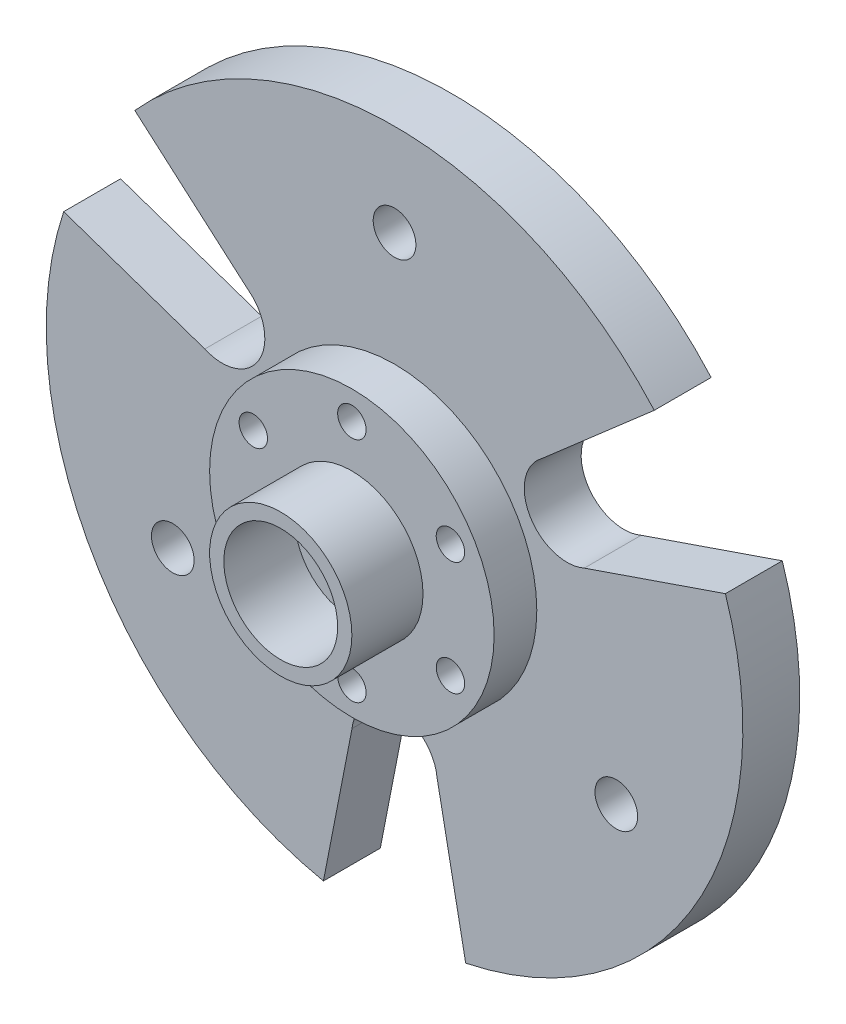
ISO-10303-21;
HEADER;
FILE_DESCRIPTION(('STEP AP214'),'2;1');
FILE_NAME('part.step','',(''),(''),'','','');
FILE_SCHEMA(('AUTOMOTIVE_DESIGN { 1 0 10303 214 1 1 1 1 }'));
ENDSEC;
DATA;
#1=APPLICATION_CONTEXT('core data for automotive mechanical design processes');
#2=APPLICATION_PROTOCOL_DEFINITION('international standard','automotive_design',2000,#1);
#3=PRODUCT_CONTEXT('',#1,'mechanical');
#4=PRODUCT('Part','Part','',(#3));
#5=PRODUCT_RELATED_PRODUCT_CATEGORY('part','',(#4));
#6=PRODUCT_DEFINITION_FORMATION('','',#4);
#7=PRODUCT_DEFINITION_CONTEXT('part definition',#1,'design');
#8=PRODUCT_DEFINITION('design','',#6,#7);
#9=PRODUCT_DEFINITION_SHAPE('','',#8);
#10=(LENGTH_UNIT() NAMED_UNIT(*) SI_UNIT(.MILLI.,.METRE.));
#11=(NAMED_UNIT(*) PLANE_ANGLE_UNIT() SI_UNIT($,.RADIAN.));
#12=(NAMED_UNIT(*) SI_UNIT($,.STERADIAN.) SOLID_ANGLE_UNIT());
#13=UNCERTAINTY_MEASURE_WITH_UNIT(LENGTH_MEASURE(1.E-05),#10,'distance_accuracy_value','');
#14=(GEOMETRIC_REPRESENTATION_CONTEXT(3) GLOBAL_UNCERTAINTY_ASSIGNED_CONTEXT((#13)) GLOBAL_UNIT_ASSIGNED_CONTEXT((#10,
#11,#12)) REPRESENTATION_CONTEXT('',''));
#15=CARTESIAN_POINT('',(0.,0.,0.));
#16=DIRECTION('',(0.,0.,1.));
#17=DIRECTION('',(1.,0.,0.));
#18=AXIS2_PLACEMENT_3D('',#15,#16,#17);
#19=CARTESIAN_POINT('',(0.,0.,4.));
#20=DIRECTION('',(0.,0.,-1.));
#21=DIRECTION('',(-1.,0.,0.));
#22=AXIS2_PLACEMENT_3D('',#19,#20,#21);
#23=CYLINDRICAL_SURFACE('',#22,24.4840524030431);
#24=CARTESIAN_POINT('',(0.,0.,0.));
#25=DIRECTION('',(0.,0.,1.));
#26=DIRECTION('',(1.,0.,0.));
#27=AXIS2_PLACEMENT_3D('',#24,#25,#26);
#28=CIRCLE('',#27,24.4840524030431);
#29=CARTESIAN_POINT('',(-23.256965494894,7.65391259711464,0.));
#30=VERTEX_POINT('',#29);
#31=CARTESIAN_POINT('',(-5.,-23.9680792320737,0.));
#32=VERTEX_POINT('',#31);
#33=EDGE_CURVE('E160',#30,#32,#28,.T.);
#34=ORIENTED_EDGE('',*,*,#33,.T.);
#35=DIRECTION('',(0.,0.,-1.));
#36=VECTOR('',#35,1.);
#37=CARTESIAN_POINT('',(-5.,-23.9680792320737,4.));
#38=LINE('',#37,#36);
#39=CARTESIAN_POINT('',(-5.,-23.9680792320737,4.));
#40=VERTEX_POINT('',#39);
#41=EDGE_CURVE('E50',#40,#32,#38,.T.);
#42=ORIENTED_EDGE('',*,*,#41,.F.);
#43=CARTESIAN_POINT('',(0.,0.,4.));
#44=DIRECTION('',(0.,0.,1.));
#45=DIRECTION('',(1.,0.,0.));
#46=AXIS2_PLACEMENT_3D('',#43,#44,#45);
#47=CIRCLE('',#46,24.4840524030431);
#48=CARTESIAN_POINT('',(-23.256965494894,7.65391259711464,4.));
#49=VERTEX_POINT('',#48);
#50=EDGE_CURVE('E182',#49,#40,#47,.T.);
#51=ORIENTED_EDGE('',*,*,#50,.F.);
#52=DIRECTION('',(0.,0.,-1.));
#53=VECTOR('',#52,1.);
#54=CARTESIAN_POINT('',(-23.256965494894,7.65391259711464,4.));
#55=LINE('',#54,#53);
#56=EDGE_CURVE('E156',#49,#30,#55,.T.);
#57=ORIENTED_EDGE('',*,*,#56,.T.);
#58=EDGE_LOOP('',(#34,#42,#51,#57));
#59=FACE_BOUND('',#58,.T.);
#60=ADVANCED_FACE('F39',(#59),#23,.T.);
#61=CARTESIAN_POINT('',(-2.98871438124849,-13.6772653095317,4.));
#62=DIRECTION('',(-0.981430995026809,0.191815541603613,0.));
#63=DIRECTION('',(-0.191815541603613,-0.981430995026809,0.));
#64=AXIS2_PLACEMENT_3D('',#61,#62,#63);
#65=PLANE('',#64);
#66=DIRECTION('',(0.191815541603613,0.981430995026809,0.));
#67=VECTOR('',#66,1.);
#68=CARTESIAN_POINT('',(-2.98871438124849,-13.6772653095317,0.));
#69=LINE('',#68,#67);
#70=CARTESIAN_POINT('',(-2.98871438124849,-13.6772653095317,0.));
#71=VERTEX_POINT('',#70);
#72=EDGE_CURVE('E161',#32,#71,#69,.T.);
#73=ORIENTED_EDGE('',*,*,#72,.T.);
#74=DIRECTION('',(0.,0.,-1.));
#75=VECTOR('',#74,1.);
#76=CARTESIAN_POINT('',(-2.98871438124849,-13.6772653095317,4.));
#77=LINE('',#76,#75);
#78=CARTESIAN_POINT('',(-2.98871438124849,-13.6772653095317,4.));
#79=VERTEX_POINT('',#78);
#80=EDGE_CURVE('E205',#79,#71,#77,.T.);
#81=ORIENTED_EDGE('',*,*,#80,.F.);
#82=DIRECTION('',(0.191815541603613,0.981430995026809,0.));
#83=VECTOR('',#82,1.);
#84=CARTESIAN_POINT('',(-2.98871438124849,-13.6772653095317,4.));
#85=LINE('',#84,#83);
#86=EDGE_CURVE('E111',#40,#79,#85,.T.);
#87=ORIENTED_EDGE('',*,*,#86,.F.);
#88=ORIENTED_EDGE('',*,*,#41,.T.);
#89=EDGE_LOOP('',(#73,#81,#87,#88));
#90=FACE_BOUND('',#89,.T.);
#91=ADVANCED_FACE('F206',(#90),#65,.F.);
#92=CARTESIAN_POINT('',(0.,-14.,4.));
#93=DIRECTION('',(0.,0.,-1.));
#94=DIRECTION('',(-1.,0.,0.));
#95=AXIS2_PLACEMENT_3D('',#92,#93,#94);
#96=CYLINDRICAL_SURFACE('',#95,3.00608904277855);
#97=CARTESIAN_POINT('',(0.,-14.,0.));
#98=DIRECTION('',(0.,0.,-1.));
#99=DIRECTION('',(1.,0.,0.));
#100=AXIS2_PLACEMENT_3D('',#97,#98,#99);
#101=CIRCLE('',#100,3.00608904277855);
#102=CARTESIAN_POINT('',(2.98871438124849,-13.6772653095317,0.));
#103=VERTEX_POINT('',#102);
#104=EDGE_CURVE('E168',#71,#103,#101,.T.);
#105=ORIENTED_EDGE('',*,*,#104,.T.);
#106=DIRECTION('',(0.,0.,-1.));
#107=VECTOR('',#106,1.);
#108=CARTESIAN_POINT('',(2.98871438124849,-13.6772653095317,4.));
#109=LINE('',#108,#107);
#110=CARTESIAN_POINT('',(2.98871438124849,-13.6772653095317,4.));
#111=VERTEX_POINT('',#110);
#112=EDGE_CURVE('E202',#111,#103,#109,.T.);
#113=ORIENTED_EDGE('',*,*,#112,.F.);
#114=CARTESIAN_POINT('',(0.,-14.,4.));
#115=DIRECTION('',(0.,0.,-1.));
#116=DIRECTION('',(1.,0.,0.));
#117=AXIS2_PLACEMENT_3D('',#114,#115,#116);
#118=CIRCLE('',#117,3.00608904277855);
#119=EDGE_CURVE('E226',#79,#111,#118,.T.);
#120=ORIENTED_EDGE('',*,*,#119,.F.);
#121=ORIENTED_EDGE('',*,*,#80,.T.);
#122=EDGE_LOOP('',(#105,#113,#120,#121));
#123=FACE_BOUND('',#122,.T.);
#124=ADVANCED_FACE('F217',(#123),#96,.F.);
#125=CARTESIAN_POINT('',(2.98871438124849,-13.6772653095317,4.));
#126=DIRECTION('',(0.981430995026809,0.191815541603613,0.));
#127=DIRECTION('',(-0.191815541603613,0.981430995026809,0.));
#128=AXIS2_PLACEMENT_3D('',#125,#126,#127);
#129=PLANE('',#128);
#130=DIRECTION('',(0.191815541603613,-0.981430995026809,0.));
#131=VECTOR('',#130,1.);
#132=CARTESIAN_POINT('',(2.98871438124849,-13.6772653095317,0.));
#133=LINE('',#132,#131);
#134=CARTESIAN_POINT('',(4.99999999999998,-23.9680792320737,0.));
#135=VERTEX_POINT('',#134);
#136=EDGE_CURVE('E166',#103,#135,#133,.T.);
#137=ORIENTED_EDGE('',*,*,#136,.T.);
#138=DIRECTION('',(0.,0.,-1.));
#139=VECTOR('',#138,1.);
#140=CARTESIAN_POINT('',(4.99999999999998,-23.9680792320737,4.));
#141=LINE('',#140,#139);
#142=CARTESIAN_POINT('',(4.99999999999998,-23.9680792320737,4.));
#143=VERTEX_POINT('',#142);
#144=EDGE_CURVE('E197',#143,#135,#141,.T.);
#145=ORIENTED_EDGE('',*,*,#144,.F.);
#146=DIRECTION('',(0.191815541603613,-0.981430995026809,0.));
#147=VECTOR('',#146,1.);
#148=CARTESIAN_POINT('',(2.98871438124849,-13.6772653095317,4.));
#149=LINE('',#148,#147);
#150=EDGE_CURVE('E225',#111,#143,#149,.T.);
#151=ORIENTED_EDGE('',*,*,#150,.F.);
#152=ORIENTED_EDGE('',*,*,#112,.T.);
#153=EDGE_LOOP('',(#137,#145,#151,#152));
#154=FACE_BOUND('',#153,.T.);
#155=ADVANCED_FACE('F224',(#154),#129,.F.);
#156=CARTESIAN_POINT('',(0.,0.,4.));
#157=DIRECTION('',(0.,0.,-1.));
#158=DIRECTION('',(-1.,0.,0.));
#159=AXIS2_PLACEMENT_3D('',#156,#157,#158);
#160=CYLINDRICAL_SURFACE('',#159,24.4840524030431);
#161=CARTESIAN_POINT('',(0.,0.,0.));
#162=DIRECTION('',(0.,0.,1.));
#163=DIRECTION('',(1.,0.,0.));
#164=AXIS2_PLACEMENT_3D('',#161,#162,#163);
#165=CIRCLE('',#164,24.4840524030431);
#166=CARTESIAN_POINT('',(23.256965494894,7.65391259711465,0.));
#167=VERTEX_POINT('',#166);
#168=EDGE_CURVE('E167',#135,#167,#165,.T.);
#169=ORIENTED_EDGE('',*,*,#168,.T.);
#170=DIRECTION('',(0.,0.,-1.));
#171=VECTOR('',#170,1.);
#172=CARTESIAN_POINT('',(23.256965494894,7.65391259711465,4.));
#173=LINE('',#172,#171);
#174=CARTESIAN_POINT('',(23.256965494894,7.65391259711465,4.));
#175=VERTEX_POINT('',#174);
#176=EDGE_CURVE('E196',#175,#167,#173,.T.);
#177=ORIENTED_EDGE('',*,*,#176,.F.);
#178=CARTESIAN_POINT('',(0.,0.,4.));
#179=DIRECTION('',(0.,0.,1.));
#180=DIRECTION('',(1.,0.,0.));
#181=AXIS2_PLACEMENT_3D('',#178,#179,#180);
#182=CIRCLE('',#181,24.4840524030431);
#183=EDGE_CURVE('E227',#143,#175,#182,.T.);
#184=ORIENTED_EDGE('',*,*,#183,.F.);
#185=ORIENTED_EDGE('',*,*,#144,.T.);
#186=EDGE_LOOP('',(#169,#177,#184,#185));
#187=FACE_BOUND('',#186,.T.);
#188=ADVANCED_FACE('F256',(#187),#160,.T.);
#189=CARTESIAN_POINT('',(13.3392164029783,4.25033007594875,4.));
#190=DIRECTION('',(0.324598365644005,-0.945851944556462,0.));
#191=DIRECTION('',(0.945851944556462,0.324598365644005,0.));
#192=AXIS2_PLACEMENT_3D('',#189,#190,#191);
#193=PLANE('',#192);
#194=DIRECTION('',(-0.945851944556462,-0.324598365644005,0.));
#195=VECTOR('',#194,1.);
#196=CARTESIAN_POINT('',(13.3392164029783,4.25033007594875,0.));
#197=LINE('',#196,#195);
#198=CARTESIAN_POINT('',(13.3392164029784,4.25033007594862,0.));
#199=VERTEX_POINT('',#198);
#200=EDGE_CURVE('E175',#167,#199,#197,.T.);
#201=ORIENTED_EDGE('',*,*,#200,.T.);
#202=DIRECTION('',(0.,0.,-1.));
#203=VECTOR('',#202,1.);
#204=CARTESIAN_POINT('',(13.3392164029784,4.25033007594862,4.));
#205=LINE('',#204,#203);
#206=CARTESIAN_POINT('',(13.3392164029784,4.25033007594862,4.));
#207=VERTEX_POINT('',#206);
#208=EDGE_CURVE('E194',#207,#199,#205,.T.);
#209=ORIENTED_EDGE('',*,*,#208,.F.);
#210=DIRECTION('',(-0.945851944556462,-0.324598365644005,0.));
#211=VECTOR('',#210,1.);
#212=CARTESIAN_POINT('',(13.3392164029783,4.25033007594875,4.));
#213=LINE('',#212,#211);
#214=EDGE_CURVE('E229',#175,#207,#213,.T.);
#215=ORIENTED_EDGE('',*,*,#214,.F.);
#216=ORIENTED_EDGE('',*,*,#176,.T.);
#217=EDGE_LOOP('',(#201,#209,#215,#216));
#218=FACE_BOUND('',#217,.T.);
#219=ADVANCED_FACE('F257',(#218),#193,.F.);
#220=CARTESIAN_POINT('',(12.1243556529822,6.99999999999989,4.));
#221=DIRECTION('',(0.,0.,-1.));
#222=DIRECTION('',(-1.,0.,0.));
#223=AXIS2_PLACEMENT_3D('',#220,#221,#222);
#224=CYLINDRICAL_SURFACE('',#223,3.00608904277855);
#225=CARTESIAN_POINT('',(12.1243556529822,6.99999999999989,0.));
#226=DIRECTION('',(0.,0.,-1.));
#227=DIRECTION('',(1.,0.,0.));
#228=AXIS2_PLACEMENT_3D('',#225,#226,#227);
#229=CIRCLE('',#228,3.00608904277855);
#230=CARTESIAN_POINT('',(10.3505020217298,9.42693523358292,0.));
#231=VERTEX_POINT('',#230);
#232=EDGE_CURVE('E172',#199,#231,#229,.T.);
#233=ORIENTED_EDGE('',*,*,#232,.T.);
#234=DIRECTION('',(0.,0.,-1.));
#235=VECTOR('',#234,1.);
#236=CARTESIAN_POINT('',(10.3505020217298,9.42693523358292,4.));
#237=LINE('',#236,#235);
#238=CARTESIAN_POINT('',(10.3505020217298,9.42693523358292,4.));
#239=VERTEX_POINT('',#238);
#240=EDGE_CURVE('E188',#239,#231,#237,.T.);
#241=ORIENTED_EDGE('',*,*,#240,.F.);
#242=CARTESIAN_POINT('',(12.1243556529822,6.99999999999989,4.));
#243=DIRECTION('',(0.,0.,-1.));
#244=DIRECTION('',(1.,0.,0.));
#245=AXIS2_PLACEMENT_3D('',#242,#243,#244);
#246=CIRCLE('',#245,3.00608904277855);
#247=EDGE_CURVE('E236',#207,#239,#246,.T.);
#248=ORIENTED_EDGE('',*,*,#247,.F.);
#249=ORIENTED_EDGE('',*,*,#208,.T.);
#250=EDGE_LOOP('',(#233,#241,#248,#249));
#251=FACE_BOUND('',#250,.T.);
#252=ADVANCED_FACE('F255',(#251),#224,.F.);
#253=CARTESIAN_POINT('',(10.3505020217298,9.42693523358292,4.));
#254=DIRECTION('',(-0.656832629382805,0.754036402952849,0.));
#255=DIRECTION('',(-0.754036402952849,-0.656832629382805,0.));
#256=AXIS2_PLACEMENT_3D('',#253,#254,#255);
#257=PLANE('',#256);
#258=DIRECTION('',(0.754036402952849,0.656832629382805,0.));
#259=VECTOR('',#258,1.);
#260=CARTESIAN_POINT('',(10.3505020217298,9.42693523358292,0.));
#261=LINE('',#260,#259);
#262=CARTESIAN_POINT('',(18.256965494894,16.314166634959,0.));
#263=VERTEX_POINT('',#262);
#264=EDGE_CURVE('E176',#231,#263,#261,.T.);
#265=ORIENTED_EDGE('',*,*,#264,.T.);
#266=DIRECTION('',(0.,0.,-1.));
#267=VECTOR('',#266,1.);
#268=CARTESIAN_POINT('',(18.256965494894,16.314166634959,4.));
#269=LINE('',#268,#267);
#270=CARTESIAN_POINT('',(18.256965494894,16.314166634959,4.));
#271=VERTEX_POINT('',#270);
#272=EDGE_CURVE('E190',#271,#263,#269,.T.);
#273=ORIENTED_EDGE('',*,*,#272,.F.);
#274=DIRECTION('',(0.754036402952849,0.656832629382805,0.));
#275=VECTOR('',#274,1.);
#276=CARTESIAN_POINT('',(10.3505020217298,9.42693523358292,4.));
#277=LINE('',#276,#275);
#278=EDGE_CURVE('E238',#239,#271,#277,.T.);
#279=ORIENTED_EDGE('',*,*,#278,.F.);
#280=ORIENTED_EDGE('',*,*,#240,.T.);
#281=EDGE_LOOP('',(#265,#273,#279,#280));
#282=FACE_BOUND('',#281,.T.);
#283=ADVANCED_FACE('F242',(#282),#257,.F.);
#284=CARTESIAN_POINT('',(0.,0.,4.));
#285=DIRECTION('',(0.,0.,-1.));
#286=DIRECTION('',(-1.,0.,0.));
#287=AXIS2_PLACEMENT_3D('',#284,#285,#286);
#288=CYLINDRICAL_SURFACE('',#287,24.4840524030431);
#289=CARTESIAN_POINT('',(0.,0.,0.));
#290=DIRECTION('',(0.,0.,1.));
#291=DIRECTION('',(1.,0.,0.));
#292=AXIS2_PLACEMENT_3D('',#289,#290,#291);
#293=CIRCLE('',#292,24.4840524030431);
#294=CARTESIAN_POINT('',(-18.256965494894,16.314166634959,0.));
#295=VERTEX_POINT('',#294);
#296=EDGE_CURVE('E178',#263,#295,#293,.T.);
#297=ORIENTED_EDGE('',*,*,#296,.T.);
#298=DIRECTION('',(0.,0.,-1.));
#299=VECTOR('',#298,1.);
#300=CARTESIAN_POINT('',(-18.256965494894,16.314166634959,4.));
#301=LINE('',#300,#299);
#302=CARTESIAN_POINT('',(-18.256965494894,16.314166634959,4.));
#303=VERTEX_POINT('',#302);
#304=EDGE_CURVE('E151',#303,#295,#301,.T.);
#305=ORIENTED_EDGE('',*,*,#304,.F.);
#306=CARTESIAN_POINT('',(0.,0.,4.));
#307=DIRECTION('',(0.,0.,1.));
#308=DIRECTION('',(1.,0.,0.));
#309=AXIS2_PLACEMENT_3D('',#306,#307,#308);
#310=CIRCLE('',#309,24.4840524030431);
#311=EDGE_CURVE('E145',#271,#303,#310,.T.);
#312=ORIENTED_EDGE('',*,*,#311,.F.);
#313=ORIENTED_EDGE('',*,*,#272,.T.);
#314=EDGE_LOOP('',(#297,#305,#312,#313));
#315=FACE_BOUND('',#314,.T.);
#316=ADVANCED_FACE('F247',(#315),#288,.T.);
#317=CARTESIAN_POINT('',(-10.3505020217298,9.42693523358292,4.));
#318=DIRECTION('',(0.656832629382805,0.754036402952849,0.));
#319=DIRECTION('',(-0.754036402952849,0.656832629382805,0.));
#320=AXIS2_PLACEMENT_3D('',#317,#318,#319);
#321=PLANE('',#320);
#322=DIRECTION('',(0.754036402952849,-0.656832629382805,0.));
#323=VECTOR('',#322,1.);
#324=CARTESIAN_POINT('',(-10.3505020217298,9.42693523358292,0.));
#325=LINE('',#324,#323);
#326=CARTESIAN_POINT('',(-10.3505020217298,9.42693523358297,0.));
#327=VERTEX_POINT('',#326);
#328=EDGE_CURVE('E148',#295,#327,#325,.T.);
#329=ORIENTED_EDGE('',*,*,#328,.T.);
#330=DIRECTION('',(0.,0.,-1.));
#331=VECTOR('',#330,1.);
#332=CARTESIAN_POINT('',(-10.3505020217298,9.42693523358297,4.));
#333=LINE('',#332,#331);
#334=CARTESIAN_POINT('',(-10.3505020217298,9.42693523358297,4.));
#335=VERTEX_POINT('',#334);
#336=EDGE_CURVE('E150',#335,#327,#333,.T.);
#337=ORIENTED_EDGE('',*,*,#336,.F.);
#338=DIRECTION('',(0.754036402952849,-0.656832629382805,0.));
#339=VECTOR('',#338,1.);
#340=CARTESIAN_POINT('',(-10.3505020217298,9.42693523358292,4.));
#341=LINE('',#340,#339);
#342=EDGE_CURVE('E136',#303,#335,#341,.T.);
#343=ORIENTED_EDGE('',*,*,#342,.F.);
#344=ORIENTED_EDGE('',*,*,#304,.T.);
#345=EDGE_LOOP('',(#329,#337,#343,#344));
#346=FACE_BOUND('',#345,.T.);
#347=ADVANCED_FACE('F149',(#346),#321,.F.);
#348=CARTESIAN_POINT('',(-12.1243556529821,7.00000000000006,4.));
#349=DIRECTION('',(0.,0.,-1.));
#350=DIRECTION('',(-1.,0.,0.));
#351=AXIS2_PLACEMENT_3D('',#348,#349,#350);
#352=CYLINDRICAL_SURFACE('',#351,3.00608904277855);
#353=CARTESIAN_POINT('',(-12.1243556529821,7.00000000000006,0.));
#354=DIRECTION('',(0.,0.,-1.));
#355=DIRECTION('',(1.,0.,0.));
#356=AXIS2_PLACEMENT_3D('',#353,#354,#355);
#357=CIRCLE('',#356,3.00608904277855);
#358=CARTESIAN_POINT('',(-13.3392164029783,4.25033007594874,0.));
#359=VERTEX_POINT('',#358);
#360=EDGE_CURVE('E98',#327,#359,#357,.T.);
#361=ORIENTED_EDGE('',*,*,#360,.T.);
#362=DIRECTION('',(0.,0.,-1.));
#363=VECTOR('',#362,1.);
#364=CARTESIAN_POINT('',(-13.3392164029783,4.25033007594874,4.));
#365=LINE('',#364,#363);
#366=CARTESIAN_POINT('',(-13.3392164029783,4.25033007594874,4.));
#367=VERTEX_POINT('',#366);
#368=EDGE_CURVE('E155',#367,#359,#365,.T.);
#369=ORIENTED_EDGE('',*,*,#368,.F.);
#370=CARTESIAN_POINT('',(-12.1243556529821,7.00000000000006,4.));
#371=DIRECTION('',(0.,0.,-1.));
#372=DIRECTION('',(1.,0.,0.));
#373=AXIS2_PLACEMENT_3D('',#370,#371,#372);
#374=CIRCLE('',#373,3.00608904277855);
#375=EDGE_CURVE('E140',#335,#367,#374,.T.);
#376=ORIENTED_EDGE('',*,*,#375,.F.);
#377=ORIENTED_EDGE('',*,*,#336,.T.);
#378=EDGE_LOOP('',(#361,#369,#376,#377));
#379=FACE_BOUND('',#378,.T.);
#380=ADVANCED_FACE('F152',(#379),#352,.F.);
#381=CARTESIAN_POINT('',(-13.3392164029783,4.25033007594874,4.));
#382=DIRECTION('',(-0.324598365644005,-0.945851944556462,0.));
#383=DIRECTION('',(0.945851944556462,-0.324598365644005,0.));
#384=AXIS2_PLACEMENT_3D('',#381,#382,#383);
#385=PLANE('',#384);
#386=DIRECTION('',(-0.945851944556462,0.324598365644005,0.));
#387=VECTOR('',#386,1.);
#388=CARTESIAN_POINT('',(-13.3392164029783,4.25033007594874,0.));
#389=LINE('',#388,#387);
#390=EDGE_CURVE('E105',#359,#30,#389,.T.);
#391=ORIENTED_EDGE('',*,*,#390,.T.);
#392=ORIENTED_EDGE('',*,*,#56,.F.);
#393=DIRECTION('',(-0.945851944556462,0.324598365644005,0.));
#394=VECTOR('',#393,1.);
#395=CARTESIAN_POINT('',(-13.3392164029783,4.25033007594874,4.));
#396=LINE('',#395,#394);
#397=EDGE_CURVE('E54',#367,#49,#396,.T.);
#398=ORIENTED_EDGE('',*,*,#397,.F.);
#399=ORIENTED_EDGE('',*,*,#368,.T.);
#400=EDGE_LOOP('',(#391,#392,#398,#399));
#401=FACE_BOUND('',#400,.T.);
#402=ADVANCED_FACE('F335',(#401),#385,.F.);
#403=CARTESIAN_POINT('',(0.,0.,4.));
#404=DIRECTION('',(0.,0.,1.));
#405=DIRECTION('',(1.,0.,0.));
#406=AXIS2_PLACEMENT_3D('',#403,#404,#405);
#407=PLANE('',#406);
#408=CARTESIAN_POINT('',(0.,0.,4.));
#409=DIRECTION('',(0.,0.,1.));
#410=DIRECTION('',(1.,0.,0.));
#411=AXIS2_PLACEMENT_3D('',#408,#409,#410);
#412=CIRCLE('',#411,10.);
#413=CARTESIAN_POINT('',(10.,0.,4.));
#414=VERTEX_POINT('',#413);
#415=EDGE_CURVE('E626',#414,#414,#412,.F.);
#416=ORIENTED_EDGE('',*,*,#415,.T.);
#417=EDGE_LOOP('',(#416));
#418=FACE_BOUND('',#417,.T.);
#419=CARTESIAN_POINT('',(0.,18.,4.));
#420=DIRECTION('',(0.,0.,1.));
#421=DIRECTION('',(1.,0.,0.));
#422=AXIS2_PLACEMENT_3D('',#419,#420,#421);
#423=CIRCLE('',#422,1.5);
#424=CARTESIAN_POINT('',(1.5,18.,4.));
#425=VERTEX_POINT('',#424);
#426=EDGE_CURVE('E165',#425,#425,#423,.T.);
#427=ORIENTED_EDGE('',*,*,#426,.F.);
#428=EDGE_LOOP('',(#427));
#429=FACE_BOUND('',#428,.T.);
#430=CARTESIAN_POINT('',(15.5884572681199,-8.99999999999999,4.));
#431=DIRECTION('',(0.,0.,1.));
#432=DIRECTION('',(1.,0.,0.));
#433=AXIS2_PLACEMENT_3D('',#430,#431,#432);
#434=CIRCLE('',#433,1.5000000000001);
#435=CARTESIAN_POINT('',(17.08845726812,-8.99999999999999,4.));
#436=VERTEX_POINT('',#435);
#437=EDGE_CURVE('E634',#436,#436,#434,.T.);
#438=ORIENTED_EDGE('',*,*,#437,.F.);
#439=EDGE_LOOP('',(#438));
#440=FACE_BOUND('',#439,.T.);
#441=CARTESIAN_POINT('',(-15.5884572681199,-9.00000000000001,4.));
#442=DIRECTION('',(0.,0.,1.));
#443=DIRECTION('',(1.,0.,0.));
#444=AXIS2_PLACEMENT_3D('',#441,#442,#443);
#445=CIRCLE('',#444,1.50000000000017);
#446=CARTESIAN_POINT('',(-14.0884572681197,-9.00000000000001,4.));
#447=VERTEX_POINT('',#446);
#448=EDGE_CURVE('E642',#447,#447,#445,.T.);
#449=ORIENTED_EDGE('',*,*,#448,.F.);
#450=EDGE_LOOP('',(#449));
#451=FACE_BOUND('',#450,.T.);
#452=ORIENTED_EDGE('',*,*,#50,.T.);
#453=ORIENTED_EDGE('',*,*,#86,.T.);
#454=ORIENTED_EDGE('',*,*,#119,.T.);
#455=ORIENTED_EDGE('',*,*,#150,.T.);
#456=ORIENTED_EDGE('',*,*,#183,.T.);
#457=ORIENTED_EDGE('',*,*,#214,.T.);
#458=ORIENTED_EDGE('',*,*,#247,.T.);
#459=ORIENTED_EDGE('',*,*,#278,.T.);
#460=ORIENTED_EDGE('',*,*,#311,.T.);
#461=ORIENTED_EDGE('',*,*,#342,.T.);
#462=ORIENTED_EDGE('',*,*,#375,.T.);
#463=ORIENTED_EDGE('',*,*,#397,.T.);
#464=EDGE_LOOP('',(#452,#453,#454,#455,#456,#457,#458,#459,#460,#461,#462,#463));
#465=FACE_BOUND('',#464,.T.);
#466=ADVANCED_FACE('F139',(#418,#429,#440,#451,#465),#407,.T.);
#467=CARTESIAN_POINT('',(0.,0.,0.));
#468=DIRECTION('',(0.,0.,1.));
#469=DIRECTION('',(1.,0.,0.));
#470=AXIS2_PLACEMENT_3D('',#467,#468,#469);
#471=PLANE('',#470);
#472=CARTESIAN_POINT('',(0.,18.,0.));
#473=DIRECTION('',(0.,0.,1.));
#474=DIRECTION('',(1.,0.,0.));
#475=AXIS2_PLACEMENT_3D('',#472,#473,#474);
#476=CIRCLE('',#475,1.5);
#477=CARTESIAN_POINT('',(1.5,18.,0.));
#478=VERTEX_POINT('',#477);
#479=EDGE_CURVE('E635',#478,#478,#476,.T.);
#480=ORIENTED_EDGE('',*,*,#479,.T.);
#481=EDGE_LOOP('',(#480));
#482=FACE_BOUND('',#481,.T.);
#483=CARTESIAN_POINT('',(15.5884572681199,-8.99999999999999,0.));
#484=DIRECTION('',(0.,0.,1.));
#485=DIRECTION('',(1.,0.,0.));
#486=AXIS2_PLACEMENT_3D('',#483,#484,#485);
#487=CIRCLE('',#486,1.5000000000001);
#488=CARTESIAN_POINT('',(17.08845726812,-8.99999999999999,0.));
#489=VERTEX_POINT('',#488);
#490=EDGE_CURVE('E637',#489,#489,#487,.T.);
#491=ORIENTED_EDGE('',*,*,#490,.T.);
#492=EDGE_LOOP('',(#491));
#493=FACE_BOUND('',#492,.T.);
#494=CARTESIAN_POINT('',(-15.5884572681199,-9.00000000000001,0.));
#495=DIRECTION('',(0.,0.,1.));
#496=DIRECTION('',(1.,0.,0.));
#497=AXIS2_PLACEMENT_3D('',#494,#495,#496);
#498=CIRCLE('',#497,1.50000000000017);
#499=CARTESIAN_POINT('',(-14.0884572681197,-9.00000000000001,0.));
#500=VERTEX_POINT('',#499);
#501=EDGE_CURVE('E627',#500,#500,#498,.T.);
#502=ORIENTED_EDGE('',*,*,#501,.T.);
#503=EDGE_LOOP('',(#502));
#504=FACE_BOUND('',#503,.T.);
#505=ORIENTED_EDGE('',*,*,#33,.F.);
#506=ORIENTED_EDGE('',*,*,#390,.F.);
#507=ORIENTED_EDGE('',*,*,#360,.F.);
#508=ORIENTED_EDGE('',*,*,#328,.F.);
#509=ORIENTED_EDGE('',*,*,#296,.F.);
#510=ORIENTED_EDGE('',*,*,#264,.F.);
#511=ORIENTED_EDGE('',*,*,#232,.F.);
#512=ORIENTED_EDGE('',*,*,#200,.F.);
#513=ORIENTED_EDGE('',*,*,#168,.F.);
#514=ORIENTED_EDGE('',*,*,#136,.F.);
#515=ORIENTED_EDGE('',*,*,#104,.F.);
#516=ORIENTED_EDGE('',*,*,#72,.F.);
#517=EDGE_LOOP('',(#505,#506,#507,#508,#509,#510,#511,#512,#513,#514,#515,#516));
#518=FACE_BOUND('',#517,.T.);
#519=ADVANCED_FACE('F214',(#482,#493,#504,#518),#471,.F.);
#520=CARTESIAN_POINT('',(-15.5884572681199,-9.00000000000001,4.));
#521=DIRECTION('',(0.,0.,-1.));
#522=DIRECTION('',(-1.,0.,0.));
#523=AXIS2_PLACEMENT_3D('',#520,#521,#522);
#524=CYLINDRICAL_SURFACE('',#523,1.50000000000017);
#525=ORIENTED_EDGE('',*,*,#448,.T.);
#526=EDGE_LOOP('',(#525));
#527=FACE_BOUND('',#526,.T.);
#528=ORIENTED_EDGE('',*,*,#501,.F.);
#529=EDGE_LOOP('',(#528));
#530=FACE_BOUND('',#529,.T.);
#531=ADVANCED_FACE('F361',(#527,#530),#524,.F.);
#532=CARTESIAN_POINT('',(15.5884572681199,-8.99999999999999,4.));
#533=DIRECTION('',(0.,0.,-1.));
#534=DIRECTION('',(-1.,0.,0.));
#535=AXIS2_PLACEMENT_3D('',#532,#533,#534);
#536=CYLINDRICAL_SURFACE('',#535,1.5000000000001);
#537=ORIENTED_EDGE('',*,*,#437,.T.);
#538=EDGE_LOOP('',(#537));
#539=FACE_BOUND('',#538,.T.);
#540=ORIENTED_EDGE('',*,*,#490,.F.);
#541=EDGE_LOOP('',(#540));
#542=FACE_BOUND('',#541,.T.);
#543=ADVANCED_FACE('F373',(#539,#542),#536,.F.);
#544=CARTESIAN_POINT('',(0.,18.,4.));
#545=DIRECTION('',(0.,0.,-1.));
#546=DIRECTION('',(-1.,0.,0.));
#547=AXIS2_PLACEMENT_3D('',#544,#545,#546);
#548=CYLINDRICAL_SURFACE('',#547,1.5);
#549=ORIENTED_EDGE('',*,*,#426,.T.);
#550=EDGE_LOOP('',(#549));
#551=FACE_BOUND('',#550,.T.);
#552=ORIENTED_EDGE('',*,*,#479,.F.);
#553=EDGE_LOOP('',(#552));
#554=FACE_BOUND('',#553,.T.);
#555=ADVANCED_FACE('F384',(#551,#554),#548,.F.);
#556=CARTESIAN_POINT('',(0.,0.,7.));
#557=DIRECTION('',(0.,0.,-1.));
#558=DIRECTION('',(-1.,0.,0.));
#559=AXIS2_PLACEMENT_3D('',#556,#557,#558);
#560=CYLINDRICAL_SURFACE('',#559,10.);
#561=ORIENTED_EDGE('',*,*,#415,.F.);
#562=EDGE_LOOP('',(#561));
#563=FACE_BOUND('',#562,.T.);
#564=CARTESIAN_POINT('',(0.,0.,7.));
#565=DIRECTION('',(0.,0.,1.));
#566=DIRECTION('',(1.,0.,0.));
#567=AXIS2_PLACEMENT_3D('',#564,#565,#566);
#568=CIRCLE('',#567,10.);
#569=CARTESIAN_POINT('',(10.,0.,7.));
#570=VERTEX_POINT('',#569);
#571=EDGE_CURVE('E595',#570,#570,#568,.T.);
#572=ORIENTED_EDGE('',*,*,#571,.F.);
#573=EDGE_LOOP('',(#572));
#574=FACE_BOUND('',#573,.T.);
#575=ADVANCED_FACE('F395',(#563,#574),#560,.T.);
#576=CARTESIAN_POINT('',(0.,0.,7.));
#577=DIRECTION('',(0.,0.,1.));
#578=DIRECTION('',(1.,0.,0.));
#579=AXIS2_PLACEMENT_3D('',#576,#577,#578);
#580=PLANE('',#579);
#581=CARTESIAN_POINT('',(0.,0.,7.));
#582=DIRECTION('',(0.,0.,1.));
#583=DIRECTION('',(1.,0.,0.));
#584=AXIS2_PLACEMENT_3D('',#581,#582,#583);
#585=CIRCLE('',#584,5.);
#586=CARTESIAN_POINT('',(5.,0.,7.));
#587=VERTEX_POINT('',#586);
#588=EDGE_CURVE('E576',#587,#587,#585,.T.);
#589=ORIENTED_EDGE('',*,*,#588,.F.);
#590=EDGE_LOOP('',(#589));
#591=FACE_BOUND('',#590,.T.);
#592=CARTESIAN_POINT('',(0.,8.,7.));
#593=DIRECTION('',(0.,0.,1.));
#594=DIRECTION('',(1.,0.,0.));
#595=AXIS2_PLACEMENT_3D('',#592,#593,#594);
#596=CIRCLE('',#595,1.);
#597=CARTESIAN_POINT('',(1.,8.,7.));
#598=VERTEX_POINT('',#597);
#599=EDGE_CURVE('E588',#598,#598,#596,.T.);
#600=ORIENTED_EDGE('',*,*,#599,.F.);
#601=EDGE_LOOP('',(#600));
#602=FACE_BOUND('',#601,.T.);
#603=CARTESIAN_POINT('',(-6.92770323027546,3.9991339745963,7.));
#604=DIRECTION('',(0.,0.,1.));
#605=DIRECTION('',(1.,0.,0.));
#606=AXIS2_PLACEMENT_3D('',#603,#604,#605);
#607=CIRCLE('',#606,1.);
#608=CARTESIAN_POINT('',(-5.92770323027546,3.9991339745963,7.));
#609=VERTEX_POINT('',#608);
#610=EDGE_CURVE('E586',#609,#609,#607,.T.);
#611=ORIENTED_EDGE('',*,*,#610,.F.);
#612=EDGE_LOOP('',(#611));
#613=FACE_BOUND('',#612,.T.);
#614=CARTESIAN_POINT('',(-6.92670323027555,-4.00086602540372,7.));
#615=DIRECTION('',(0.,0.,1.));
#616=DIRECTION('',(1.,0.,0.));
#617=AXIS2_PLACEMENT_3D('',#614,#615,#616);
#618=CIRCLE('',#617,1.);
#619=CARTESIAN_POINT('',(-5.92670323027555,-4.00086602540372,7.));
#620=VERTEX_POINT('',#619);
#621=EDGE_CURVE('E602',#620,#620,#618,.T.);
#622=ORIENTED_EDGE('',*,*,#621,.F.);
#623=EDGE_LOOP('',(#622));
#624=FACE_BOUND('',#623,.T.);
#625=CARTESIAN_POINT('',(0.00199999999994414,-8.,7.));
#626=DIRECTION('',(0.,0.,1.));
#627=DIRECTION('',(1.,0.,0.));
#628=AXIS2_PLACEMENT_3D('',#625,#626,#627);
#629=CIRCLE('',#628,1.);
#630=CARTESIAN_POINT('',(1.00199999999994,-8.,7.));
#631=VERTEX_POINT('',#630);
#632=EDGE_CURVE('E613',#631,#631,#629,.T.);
#633=ORIENTED_EDGE('',*,*,#632,.F.);
#634=EDGE_LOOP('',(#633));
#635=FACE_BOUND('',#634,.T.);
#636=CARTESIAN_POINT('',(6.92970323027549,-3.99913397459625,7.));
#637=DIRECTION('',(0.,0.,1.));
#638=DIRECTION('',(1.,0.,0.));
#639=AXIS2_PLACEMENT_3D('',#636,#637,#638);
#640=CIRCLE('',#639,1.);
#641=CARTESIAN_POINT('',(7.92970323027549,-3.99913397459625,7.));
#642=VERTEX_POINT('',#641);
#643=EDGE_CURVE('E608',#642,#642,#640,.T.);
#644=ORIENTED_EDGE('',*,*,#643,.F.);
#645=EDGE_LOOP('',(#644));
#646=FACE_BOUND('',#645,.T.);
#647=CARTESIAN_POINT('',(6.92870323027552,4.00086602540377,7.));
#648=DIRECTION('',(0.,0.,1.));
#649=DIRECTION('',(1.,0.,0.));
#650=AXIS2_PLACEMENT_3D('',#647,#648,#649);
#651=CIRCLE('',#650,1.);
#652=CARTESIAN_POINT('',(7.92870323027552,4.00086602540377,7.));
#653=VERTEX_POINT('',#652);
#654=EDGE_CURVE('E605',#653,#653,#651,.T.);
#655=ORIENTED_EDGE('',*,*,#654,.F.);
#656=EDGE_LOOP('',(#655));
#657=FACE_BOUND('',#656,.T.);
#658=ORIENTED_EDGE('',*,*,#571,.T.);
#659=EDGE_LOOP('',(#658));
#660=FACE_BOUND('',#659,.T.);
#661=ADVANCED_FACE('F402',(#591,#602,#613,#624,#635,#646,#657,#660),#580,.T.);
#662=CARTESIAN_POINT('',(6.92870323027552,4.00086602540377,1.17157287525381));
#663=DIRECTION('',(0.,0.,1.));
#664=DIRECTION('',(1.,0.,0.));
#665=AXIS2_PLACEMENT_3D('',#662,#663,#664);
#666=CYLINDRICAL_SURFACE('',#665,1.);
#667=CARTESIAN_POINT('',(6.92870323027552,4.00086602540377,4.));
#668=DIRECTION('',(0.,0.,1.));
#669=DIRECTION('',(1.,0.,0.));
#670=AXIS2_PLACEMENT_3D('',#667,#668,#669);
#671=CIRCLE('',#670,1.);
#672=CARTESIAN_POINT('',(7.92870323027552,4.00086602540377,4.));
#673=VERTEX_POINT('',#672);
#674=EDGE_CURVE('E592',#673,#673,#671,.F.);
#675=ORIENTED_EDGE('',*,*,#674,.T.);
#676=EDGE_LOOP('',(#675));
#677=FACE_BOUND('',#676,.T.);
#678=ORIENTED_EDGE('',*,*,#654,.T.);
#679=EDGE_LOOP('',(#678));
#680=FACE_BOUND('',#679,.T.);
#681=ADVANCED_FACE('F415',(#677,#680),#666,.F.);
#682=CARTESIAN_POINT('',(0.,0.,4.));
#683=DIRECTION('',(0.,0.,1.));
#684=DIRECTION('',(1.,0.,0.));
#685=AXIS2_PLACEMENT_3D('',#682,#683,#684);
#686=PLANE('',#685);
#687=ORIENTED_EDGE('',*,*,#674,.F.);
#688=EDGE_LOOP('',(#687));
#689=FACE_BOUND('',#688,.T.);
#690=ADVANCED_FACE('F425',(#689),#686,.T.);
#691=CARTESIAN_POINT('',(6.92970323027549,-3.99913397459625,1.17157287525381));
#692=DIRECTION('',(0.,0.,1.));
#693=DIRECTION('',(1.,0.,0.));
#694=AXIS2_PLACEMENT_3D('',#691,#692,#693);
#695=CYLINDRICAL_SURFACE('',#694,1.);
#696=CARTESIAN_POINT('',(6.92970323027549,-3.99913397459625,4.));
#697=DIRECTION('',(0.,0.,1.));
#698=DIRECTION('',(1.,0.,0.));
#699=AXIS2_PLACEMENT_3D('',#696,#697,#698);
#700=CIRCLE('',#699,1.);
#701=CARTESIAN_POINT('',(7.92970323027549,-3.99913397459625,4.));
#702=VERTEX_POINT('',#701);
#703=EDGE_CURVE('E603',#702,#702,#700,.F.);
#704=ORIENTED_EDGE('',*,*,#703,.T.);
#705=EDGE_LOOP('',(#704));
#706=FACE_BOUND('',#705,.T.);
#707=ORIENTED_EDGE('',*,*,#643,.T.);
#708=EDGE_LOOP('',(#707));
#709=FACE_BOUND('',#708,.T.);
#710=ADVANCED_FACE('F432',(#706,#709),#695,.F.);
#711=CARTESIAN_POINT('',(0.,0.,4.));
#712=DIRECTION('',(0.,0.,1.));
#713=DIRECTION('',(1.,0.,0.));
#714=AXIS2_PLACEMENT_3D('',#711,#712,#713);
#715=PLANE('',#714);
#716=ORIENTED_EDGE('',*,*,#703,.F.);
#717=EDGE_LOOP('',(#716));
#718=FACE_BOUND('',#717,.T.);
#719=ADVANCED_FACE('F443',(#718),#715,.T.);
#720=CARTESIAN_POINT('',(0.00199999999994414,-8.,1.17157287525381));
#721=DIRECTION('',(0.,0.,1.));
#722=DIRECTION('',(1.,0.,0.));
#723=AXIS2_PLACEMENT_3D('',#720,#721,#722);
#724=CYLINDRICAL_SURFACE('',#723,1.);
#725=CARTESIAN_POINT('',(0.00199999999994414,-8.,4.));
#726=DIRECTION('',(0.,0.,1.));
#727=DIRECTION('',(1.,0.,0.));
#728=AXIS2_PLACEMENT_3D('',#725,#726,#727);
#729=CIRCLE('',#728,1.);
#730=CARTESIAN_POINT('',(1.00199999999994,-8.,4.));
#731=VERTEX_POINT('',#730);
#732=EDGE_CURVE('E611',#731,#731,#729,.F.);
#733=ORIENTED_EDGE('',*,*,#732,.T.);
#734=EDGE_LOOP('',(#733));
#735=FACE_BOUND('',#734,.T.);
#736=ORIENTED_EDGE('',*,*,#632,.T.);
#737=EDGE_LOOP('',(#736));
#738=FACE_BOUND('',#737,.T.);
#739=ADVANCED_FACE('F451',(#735,#738),#724,.F.);
#740=CARTESIAN_POINT('',(0.,0.,4.));
#741=DIRECTION('',(0.,0.,1.));
#742=DIRECTION('',(1.,0.,0.));
#743=AXIS2_PLACEMENT_3D('',#740,#741,#742);
#744=PLANE('',#743);
#745=ORIENTED_EDGE('',*,*,#732,.F.);
#746=EDGE_LOOP('',(#745));
#747=FACE_BOUND('',#746,.T.);
#748=ADVANCED_FACE('F463',(#747),#744,.T.);
#749=CARTESIAN_POINT('',(-6.92670323027555,-4.00086602540372,1.17157287525381));
#750=DIRECTION('',(0.,0.,1.));
#751=DIRECTION('',(1.,0.,0.));
#752=AXIS2_PLACEMENT_3D('',#749,#750,#751);
#753=CYLINDRICAL_SURFACE('',#752,1.);
#754=CARTESIAN_POINT('',(-6.92670323027555,-4.00086602540372,4.));
#755=DIRECTION('',(0.,0.,1.));
#756=DIRECTION('',(1.,0.,0.));
#757=AXIS2_PLACEMENT_3D('',#754,#755,#756);
#758=CIRCLE('',#757,1.);
#759=CARTESIAN_POINT('',(-5.92670323027555,-4.00086602540372,4.));
#760=VERTEX_POINT('',#759);
#761=EDGE_CURVE('E617',#760,#760,#758,.F.);
#762=ORIENTED_EDGE('',*,*,#761,.T.);
#763=EDGE_LOOP('',(#762));
#764=FACE_BOUND('',#763,.T.);
#765=ORIENTED_EDGE('',*,*,#621,.T.);
#766=EDGE_LOOP('',(#765));
#767=FACE_BOUND('',#766,.T.);
#768=ADVANCED_FACE('F471',(#764,#767),#753,.F.);
#769=CARTESIAN_POINT('',(0.,0.,4.));
#770=DIRECTION('',(0.,0.,1.));
#771=DIRECTION('',(1.,0.,0.));
#772=AXIS2_PLACEMENT_3D('',#769,#770,#771);
#773=PLANE('',#772);
#774=ORIENTED_EDGE('',*,*,#761,.F.);
#775=EDGE_LOOP('',(#774));
#776=FACE_BOUND('',#775,.T.);
#777=ADVANCED_FACE('F483',(#776),#773,.T.);
#778=CARTESIAN_POINT('',(-6.92770323027546,3.9991339745963,1.17157287525381));
#779=DIRECTION('',(0.,0.,1.));
#780=DIRECTION('',(1.,0.,0.));
#781=AXIS2_PLACEMENT_3D('',#778,#779,#780);
#782=CYLINDRICAL_SURFACE('',#781,1.);
#783=CARTESIAN_POINT('',(-6.92770323027546,3.9991339745963,4.));
#784=DIRECTION('',(0.,0.,1.));
#785=DIRECTION('',(1.,0.,0.));
#786=AXIS2_PLACEMENT_3D('',#783,#784,#785);
#787=CIRCLE('',#786,1.);
#788=CARTESIAN_POINT('',(-5.92770323027546,3.9991339745963,4.));
#789=VERTEX_POINT('',#788);
#790=EDGE_CURVE('E596',#789,#789,#787,.F.);
#791=ORIENTED_EDGE('',*,*,#790,.T.);
#792=EDGE_LOOP('',(#791));
#793=FACE_BOUND('',#792,.T.);
#794=ORIENTED_EDGE('',*,*,#610,.T.);
#795=EDGE_LOOP('',(#794));
#796=FACE_BOUND('',#795,.T.);
#797=ADVANCED_FACE('F494',(#793,#796),#782,.F.);
#798=CARTESIAN_POINT('',(0.,0.,4.));
#799=DIRECTION('',(0.,0.,1.));
#800=DIRECTION('',(1.,0.,0.));
#801=AXIS2_PLACEMENT_3D('',#798,#799,#800);
#802=PLANE('',#801);
#803=ORIENTED_EDGE('',*,*,#790,.F.);
#804=EDGE_LOOP('',(#803));
#805=FACE_BOUND('',#804,.T.);
#806=ADVANCED_FACE('F502',(#805),#802,.T.);
#807=CARTESIAN_POINT('',(0.,8.,1.17157287525381));
#808=DIRECTION('',(0.,0.,1.));
#809=DIRECTION('',(1.,0.,0.));
#810=AXIS2_PLACEMENT_3D('',#807,#808,#809);
#811=CYLINDRICAL_SURFACE('',#810,1.);
#812=CARTESIAN_POINT('',(0.,8.,4.));
#813=DIRECTION('',(0.,0.,1.));
#814=DIRECTION('',(1.,0.,0.));
#815=AXIS2_PLACEMENT_3D('',#812,#813,#814);
#816=CIRCLE('',#815,1.);
#817=CARTESIAN_POINT('',(1.,8.,4.));
#818=VERTEX_POINT('',#817);
#819=EDGE_CURVE('E591',#818,#818,#816,.F.);
#820=ORIENTED_EDGE('',*,*,#819,.T.);
#821=EDGE_LOOP('',(#820));
#822=FACE_BOUND('',#821,.T.);
#823=ORIENTED_EDGE('',*,*,#599,.T.);
#824=EDGE_LOOP('',(#823));
#825=FACE_BOUND('',#824,.T.);
#826=ADVANCED_FACE('F511',(#822,#825),#811,.F.);
#827=CARTESIAN_POINT('',(0.,0.,4.));
#828=DIRECTION('',(0.,0.,1.));
#829=DIRECTION('',(1.,0.,0.));
#830=AXIS2_PLACEMENT_3D('',#827,#828,#829);
#831=PLANE('',#830);
#832=ORIENTED_EDGE('',*,*,#819,.F.);
#833=EDGE_LOOP('',(#832));
#834=FACE_BOUND('',#833,.T.);
#835=ADVANCED_FACE('F522',(#834),#831,.T.);
#836=CARTESIAN_POINT('',(0.,0.,12.));
#837=DIRECTION('',(0.,0.,1.));
#838=DIRECTION('',(1.,0.,0.));
#839=AXIS2_PLACEMENT_3D('',#836,#837,#838);
#840=PLANE('',#839);
#841=CARTESIAN_POINT('',(0.,0.,12.));
#842=DIRECTION('',(0.,0.,1.));
#843=DIRECTION('',(1.,0.,0.));
#844=AXIS2_PLACEMENT_3D('',#841,#842,#843);
#845=CIRCLE('',#844,5.);
#846=CARTESIAN_POINT('',(5.,0.,12.));
#847=VERTEX_POINT('',#846);
#848=EDGE_CURVE('E585',#847,#847,#845,.T.);
#849=ORIENTED_EDGE('',*,*,#848,.T.);
#850=EDGE_LOOP('',(#849));
#851=FACE_BOUND('',#850,.T.);
#852=CARTESIAN_POINT('',(0.,0.,12.));
#853=DIRECTION('',(0.,0.,1.));
#854=DIRECTION('',(1.,0.,0.));
#855=AXIS2_PLACEMENT_3D('',#852,#853,#854);
#856=CIRCLE('',#855,4.);
#857=CARTESIAN_POINT('',(4.,0.,12.));
#858=VERTEX_POINT('',#857);
#859=EDGE_CURVE('E577',#858,#858,#856,.T.);
#860=ORIENTED_EDGE('',*,*,#859,.F.);
#861=EDGE_LOOP('',(#860));
#862=FACE_BOUND('',#861,.T.);
#863=ADVANCED_FACE('F531',(#851,#862),#840,.T.);
#864=CARTESIAN_POINT('',(0.,0.,12.));
#865=DIRECTION('',(0.,0.,-1.));
#866=DIRECTION('',(-1.,0.,0.));
#867=AXIS2_PLACEMENT_3D('',#864,#865,#866);
#868=CYLINDRICAL_SURFACE('',#867,5.);
#869=ORIENTED_EDGE('',*,*,#848,.F.);
#870=EDGE_LOOP('',(#869));
#871=FACE_BOUND('',#870,.T.);
#872=ORIENTED_EDGE('',*,*,#588,.T.);
#873=EDGE_LOOP('',(#872));
#874=FACE_BOUND('',#873,.T.);
#875=ADVANCED_FACE('F550',(#871,#874),#868,.T.);
#876=CARTESIAN_POINT('',(0.,0.,12.));
#877=DIRECTION('',(0.,0.,-1.));
#878=DIRECTION('',(-1.,0.,0.));
#879=AXIS2_PLACEMENT_3D('',#876,#877,#878);
#880=CYLINDRICAL_SURFACE('',#879,4.);
#881=ORIENTED_EDGE('',*,*,#859,.T.);
#882=EDGE_LOOP('',(#881));
#883=FACE_BOUND('',#882,.T.);
#884=CARTESIAN_POINT('',(0.,0.,7.));
#885=DIRECTION('',(0.,0.,1.));
#886=DIRECTION('',(1.,0.,0.));
#887=AXIS2_PLACEMENT_3D('',#884,#885,#886);
#888=CIRCLE('',#887,4.);
#889=CARTESIAN_POINT('',(4.,0.,7.));
#890=VERTEX_POINT('',#889);
#891=EDGE_CURVE('E11',#890,#890,#888,.F.);
#892=ORIENTED_EDGE('',*,*,#891,.T.);
#893=EDGE_LOOP('',(#892));
#894=FACE_BOUND('',#893,.T.);
#895=ADVANCED_FACE('F543',(#883,#894),#880,.F.);
#896=ORIENTED_EDGE('',*,*,#891,.F.);
#897=EDGE_LOOP('',(#896));
#898=FACE_BOUND('',#897,.T.);
#899=ADVANCED_FACE('F414',(#898),#580,.T.);
#900=CLOSED_SHELL('',(#60,#91,#124,#155,#188,#219,#252,#283,#316,#347,#380,#402,#466,#519,#531,
#543,#555,#575,#661,#681,#690,#710,#719,#739,#748,#768,#777,#797,#806,#826,#835,#863,#875,#895,#899));
#901=MANIFOLD_SOLID_BREP('B2',#900);
#902=ADVANCED_BREP_SHAPE_REPRESENTATION('',(#18,#901),#14);
#903=SHAPE_DEFINITION_REPRESENTATION(#9,#902);
ENDSEC;
END-ISO-10303-21;
